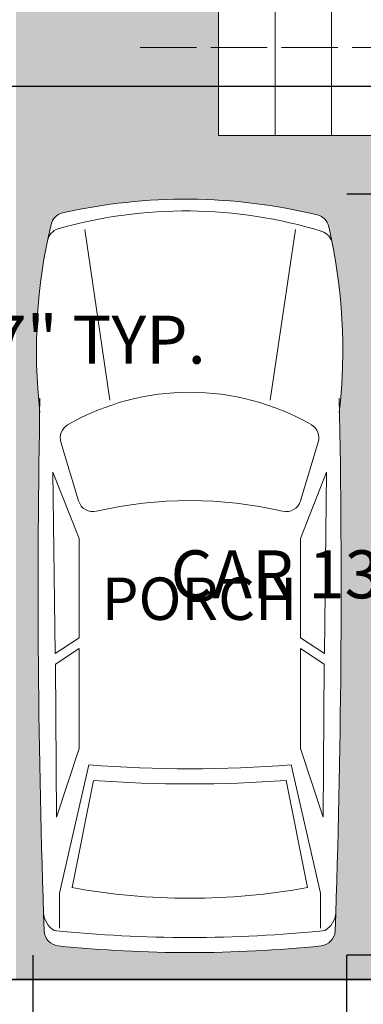
# Model space of a CAD drawing. Units: inches. Extents: x 1077 to 2505, y 1892 to 2728.
# Tile 22 of 26: x 2291 to 2364, y 2089 to 2298. Entities that reach past the tile are written whole.
import ezdxf

# ---------------------------------------------------------------- set-up
doc = ezdxf.new("R2010")
doc.units = ezdxf.units.IN
doc.linetypes.add('ACAD_ISO02W100', pattern=[15, 12, -3])
doc.layers.get('Defpoints').update_dxf_attribs({"color": 220, "linetype": 'ACAD_ISO02W100'})
for name, color, linetype, lineweight in [('A-ANNO-DIMS', 2, 'Continuous', 18), ('A-ANNO-STRS', 220, 'ACAD_ISO02W100', 13), ('A-AREA-IDEN', 7, 'Continuous', 18), ('A-FLOR-FIXT', 8, 'Continuous', 13), ('A-FLOR-STRS', 7, 'Continuous', 18), ('A-FURNITURE', 251, 'Continuous', 5), ('A-SITE-VEHI', 8, 'Continuous', 13), ('A_TEXT_SMALL', 18, 'Continuous', 13), ('WALL', 7, 'Continuous', 35)]:
    doc.layers.add(name, color=color, linetype=linetype, lineweight=lineweight)
doc.layers.add('A-FLOR-PATT', color=254, linetype='Continuous', lineweight=9, true_color=0xd7ebd2)
doc.styles.get("Standard").update_dxf_attribs({"font": 'arial.ttf'})
doc.dimstyles.get("Standard").update_dxf_attribs({"dimtxt": 10.18, "dimasz": 0.18, "dimexe": 0.18, "dimexo": 0.0625, "dimgap": 0.09, "dimtad": 0, "dimtih": 1, "dimtoh": 1, "dimdec": 0, "dimzin": 0, "dimdsep": 46, "dimlunit": 3, "dimtxsty": 'Standard', "dimcen": 0.09, "dimadec": 0, "dimazin": 0, "dimtfac": 1, "dimtdec": 0, "dimtofl": 0, "dimtmove": 0, "dimatfit": 3, "dimfxl": 1, "dimtolj": 1, "dimtzin": 0, "dimarcsym": 0})

# ---------------------------------------------------------------- blocks, each defined once
blk = doc.blocks.new('CAR')
at = {"layer": 'A-FURNITURE'}
for p, q in [((2677.91, 1665.57), (2683.24, 1629.33)), ((2722.63, 1665.57), (2717.3, 1629.33)), ((2672.85, 1620.44), (2676.61, 1608)), ((2727.48, 1620.44), (2723.73, 1608)), ((2671.15, 1614.07), (2676.73, 1600.01)), ((2671.63, 1575.61), (2671.15, 1614.07)), ((2729.25, 1614.07), (2723.67, 1600.01)), ((2728.77, 1575.61), (2729.25, 1614.07)), ((2676.73, 1600.01), (2676.73, 1578.97)), ((2723.67, 1600.01), (2723.67, 1578.97)), ((2676.73, 1578.97), (2671.63, 1575.61)), ((2723.67, 1578.97), (2728.77, 1575.61)), ((2676.73, 1576.71), (2671.66, 1573.38)), ((2676.73, 1576.71), (2676.73, 1555.46)), ((2723.67, 1576.71), (2723.67, 1555.46)), ((2723.67, 1576.71), (2728.74, 1573.38)), ((2671.9, 1540.91), (2671.66, 1573.38)), ((2728.49, 1540.91), (2728.74, 1573.38)), ((2676.73, 1555.46), (2671.9, 1540.91)), ((2723.67, 1555.46), (2728.49, 1540.91)), ((2678.77, 1552.01), (2672.52, 1524.85)), ((2721.71, 1552.02), (2727.96, 1524.85)), ((2675.22, 1526.01), (2679.74, 1548.74)), ((2725.17, 1526.01), (2720.66, 1548.74)), ((2672.52, 1524.85), (2672.52, 1517.39)), ((2727.96, 1524.85), (2727.96, 1517.39))]:
    blk.add_line(p, q, dxfattribs=at)
for centre, radius, start, end in [((2699.3, 1552.83), 119.14, 76.3976, 102.667), ((2674, 1665.84), 3.34, 104.3452, 166.6607), ((2699.3, 1570.19), 99.28, 73.0347, 105.8141), ((2726.43, 1665.41), 3.34, 13.1156, 74.5941), ((2783.1, 1639.97), 115.47, 166.6607, 186.5655), ((2617.23, 1639.97), 115.47, 353.4345, 13.1156), ((2673.27, 1662.52), 3.34, 107.8179, 168.3942), ((2727.17, 1661.99), 3.34, 11.3249, 70.8826), ((2700.17, 1579.09), 51.94, 60.0774, 119.9226), ((4741.11, 1589.62), 2073.11, 178.89024, 182.01225), ((659.22, 1589.62), 2073.11, 357.98775, 1.10976), ((2675.91, 1621.37), 3.2, 121.1455, 196.7984), ((2724.42, 1621.37), 3.2, 343.2016, 58.8545), ((2679.67, 1608.92), 3.2, 196.7984, 283.6631), ((2700.17, 1519.83), 88.22, 77.0683, 102.9317), ((2720.66, 1608.92), 3.2, 256.3369, 343.2016), ((2700.16, 1829.45), 278.26, 265.5919, 274.4407), ((2700.17, 1827.63), 279.65, 265.7971, 274.2029), ((2700.17, 1663.47), 139.72, 259.6897, 280.3103), ((2674.03, 1521.04), 4.9, 184.3987, 237.5288), ((2726.3, 1521.04), 4.9, 302.4712, 355.6013), ((2672.62, 1516.95), 3.34, 182.1119, 263.4899), ((2700.17, 1791.26), 275.86, 264.0142, 275.9858), ((2727.71, 1516.95), 3.34, 276.5101, 357.8881), ((2700.17, 1790.18), 277.96, 264.2342, 275.7658)]:
    blk.add_arc(centre, radius, start, end, dxfattribs=at)
blk = doc.blocks.new('reh-flat-2')
at = {"layer": 'A_TEXT_SMALL'}
for p, q in [((486053827.2, -394630231.2), (486054182.4, -394629799.8)), ((486054182.4, -394629799.8), (486054596.6, -394630140.9)), ((486053979.5, -394630126.3), (486054157.1, -394629910.6)), ((486054228.6, -394629903.6), (486054483.5, -394630113.5)), ((486054596.6, -394630140.9), (486054241.4, -394630572.3)), ((486054241.3, -394630407.7), (486053986.4, -394630197.8)), ((486054490.4, -394630185), (486054312.8, -394630400.7)), ((486054241.4, -394630572.3), (486053827.2, -394630231.2))]:
    blk.add_line(p, q, dxfattribs=at)
for centre, radius in [((486054234.9, -394630155.7), 38.1), ((486054004.1, -394630296.2), 20.1), ((486054072.7, -394630352.7), 20.1), ((486054141.4, -394630409.3), 20.1)]:
    blk.add_circle(centre, radius, dxfattribs=at)
for centre, start, end in [((486054196.3, -394629942.9), 50.5305, 140.5305), ((486054018.7, -394630158.5), 140.5305, 230.5305), ((486054451.2, -394630152.8), 320.5305, 50.5305), ((486054273.6, -394630368.4), 230.5305, 320.5305)]:
    blk.add_arc(centre, 50.8, start, end, dxfattribs=at)
blk = doc.blocks.new('STAIR-PLAN-RETURN')
for p, q in [((0, 163.08), (0, 127.08)), ((12, 163.08), (12, 127.08)), ((24, 163.08), (24, 127.08)), ((36, 163.08), (36, 0)), ((36, 163.08), (36, 127.08)), ((0, 127.08), (72, 127.08)), ((36, 115.08), (72, 115.08)), ((36, 103.08), (72, 103.08)), ((36, 91.08), (72, 91.08)), ((36, 79.08), (72, 79.08)), ((36, 67.08), (72, 67.08)), ((36, 55.08), (72, 55.08)), ((36, 43.08), (72, 43.08)), ((36, 31.08), (72, 31.08)), ((36, 19.08), (72, 19.08)), ((36, 7.08), (72, 7.08)), ((72, 0), (36, 0))]:
    blk.add_line(p, q)
blk = doc.blocks.new('STAIR-DIRECTION')
for p, q in [((0, 107.9), (70.51, 107.9)), ((70.51, 107.9), (70.51, 0)), ((70.51, 0), (75.75, 12.88)), ((75.75, 12.88), (70.51, 0.8)), ((70.51, 0.8), (65.28, 12.48)), ((65.28, 12.48), (70.51, 1.21))]:
    blk.add_line(p, q)
blk = doc.blocks.new('*D40')
at = {"layer": 'A-ANNO-DIMS', "color": 0, "lineweight": -2, "transparency": 16777216}
for p, q in [((2203.23, 2225.22), (2203.23, 2230.01)), ((2203.41, 2229.83), (2234.16, 2229.83)), ((2234.34, 2225.22), (2234.34, 2230.01)), ((2234.34, 2229.83), (2234.52, 2229.83))]:
    blk.add_line(p, q, dxfattribs=at)
at = {"layer": 'A-ANNO-DIMS', "color": 0, "transparency": 16777216}
for points in [[(2203.41, 2229.86), (2203.41, 2229.8), (2203.23, 2229.83)], [(2234.16, 2229.86), (2234.16, 2229.8), (2234.34, 2229.83)]]:
    blk.add_solid(points, dxfattribs=at)
at = {"layer": 'Defpoints', "color": 0, "transparency": 16777216}
for p in [(2234.34, 2229.83), (2203.23, 2225.16), (2234.34, 2225.16)]:
    blk.add_point(p, dxfattribs=at)
at = {"layer": 'A-ANNO-DIMS', "color": 0, "transparency": 16777216, "insert": (2282.74, 2229.83), "char_height": 10.18, "attachment_point": 5}
blk.add_mtext('\\A1;HOB 2\'-7" TYP.', dxfattribs=at)
blk = doc.blocks.new('*D46')
at = {"layer": 'A-ANNO-DIMS', "color": 0, "lineweight": -2, "transparency": 16777216}
for p, q in [((2289.89, 2308.17), (2289.89, 2302.65)), ((2325.89, 2308.17), (2325.89, 2302.65)), ((2289.89, 2302.83), (2289.71, 2302.83)), ((2325.71, 2302.83), (2290.07, 2302.83))]:
    blk.add_line(p, q, dxfattribs=at)
at = {"layer": 'A-ANNO-DIMS', "color": 0, "transparency": 16777216}
for points in [[(2290.07, 2302.86), (2290.07, 2302.8), (2289.89, 2302.83)], [(2325.71, 2302.86), (2325.71, 2302.8), (2325.89, 2302.83)]]:
    blk.add_solid(points, dxfattribs=at)
at = {"layer": 'Defpoints', "color": 0, "transparency": 16777216}
for p in [(2289.89, 2308.23), (2325.89, 2308.23), (2289.89, 2302.83)]:
    blk.add_point(p, dxfattribs=at)
at = {"layer": 'A-ANNO-DIMS', "color": 0, "transparency": 16777216, "insert": (2209.47, 2302.83), "char_height": 10.18, "attachment_point": 5}
blk.add_mtext('\\A1;DOOR SWING 3\'-0" TYP.', dxfattribs=at)
blk = doc.blocks.new('*D56')
at = {"layer": 'A-ANNO-DIMS', "color": 0, "lineweight": -2, "transparency": 16777216}
for p, q in [((2360.05, 2260.72), (2384.37, 2260.72)), ((2384.19, 2260.54), (2384.19, 2185.41)), ((2384.19, 2099.57), (2384.19, 2174.7)), ((2360.05, 2099.39), (2384.37, 2099.39))]:
    blk.add_line(p, q, dxfattribs=at)
at = {"layer": 'A-ANNO-DIMS', "color": 0, "transparency": 16777216}
for points in [[(2384.16, 2260.54), (2384.22, 2260.54), (2384.19, 2260.72)], [(2384.16, 2099.57), (2384.22, 2099.57), (2384.19, 2099.39)]]:
    blk.add_solid(points, dxfattribs=at)
at = {"layer": 'Defpoints', "color": 0, "transparency": 16777216}
for p in [(2359.99, 2260.72), (2384.19, 2260.72), (2359.99, 2099.39)]:
    blk.add_point(p, dxfattribs=at)
at = {"layer": 'A-ANNO-DIMS', "color": 0, "transparency": 16777216, "insert": (2384.19, 2180.06), "char_height": 10.18, "attachment_point": 5}
blk.add_mtext('\\A1;CAR 13\'-5 1/2" TYP.', dxfattribs=at)
blk = doc.blocks.new('*D57')
at = {"layer": 'A-ANNO-DIMS', "color": 0, "lineweight": -2, "transparency": 16777216}
for p, q in [((2293.39, 2099.33), (2293.39, 2075.01)), ((2359.99, 2099.33), (2359.99, 2075.01)), ((2293.57, 2075.19), (2359.81, 2075.19)), ((2359.99, 2075.19), (2360.17, 2075.19))]:
    blk.add_line(p, q, dxfattribs=at)
at = {"layer": 'A-ANNO-DIMS', "color": 0, "transparency": 16777216}
for points in [[(2293.57, 2075.22), (2293.57, 2075.16), (2293.39, 2075.19)], [(2359.81, 2075.22), (2359.81, 2075.16), (2359.99, 2075.19)]]:
    blk.add_solid(points, dxfattribs=at)
at = {"layer": 'Defpoints', "color": 0, "transparency": 16777216}
for p in [(2293.39, 2099.39), (2359.99, 2099.39), (2359.99, 2075.19)]:
    blk.add_point(p, dxfattribs=at)
at = {"layer": 'A-ANNO-DIMS', "color": 0, "transparency": 16777216, "insert": (2403.15, 2075.19), "char_height": 10.18, "attachment_point": 5}
blk.add_mtext('\\A1;5\'-6 1/2" TYP.', dxfattribs=at)
blk = doc.blocks.new('*D63')
at = {"layer": 'A-ANNO-DIMS', "color": 0, "lineweight": -2, "transparency": 16777216}
for p, q in [((2035.85, 2094.07), (2035.85, 2065.11)), ((2413.85, 2094.07), (2413.85, 2065.11)), ((2036.03, 2065.29), (2207.27, 2065.29)), ((2413.67, 2065.29), (2242.42, 2065.29))]:
    blk.add_line(p, q, dxfattribs=at)
at = {"layer": 'A-ANNO-DIMS', "color": 0, "transparency": 16777216}
for points in [[(2036.03, 2065.32), (2036.03, 2065.26), (2035.85, 2065.29)], [(2413.67, 2065.32), (2413.67, 2065.26), (2413.85, 2065.29)]]:
    blk.add_solid(points, dxfattribs=at)
at = {"layer": 'Defpoints', "color": 0, "transparency": 16777216}
for p in [(2035.85, 2094.14), (2413.85, 2094.14), (2413.85, 2065.29)]:
    blk.add_point(p, dxfattribs=at)
at = {"layer": 'A-ANNO-DIMS', "color": 0, "transparency": 16777216, "insert": (2224.85, 2065.29), "char_height": 10.18, "attachment_point": 5}
blk.add_mtext('\\A1;31\'-6"', dxfattribs=at)
blk = doc.blocks.new('*D69')
at = {"layer": 'A-ANNO-DIMS', "color": 0, "lineweight": -2, "transparency": 16777216}
for p, q in [((2263.27, 2262.49), (2263.27, 2065.11)), ((2285.18, 2262.49), (2285.18, 2065.11)), ((2263.45, 2065.29), (2285, 2065.29)), ((2285.18, 2065.29), (2285.36, 2065.29))]:
    blk.add_line(p, q, dxfattribs=at)
at = {"layer": 'A-ANNO-DIMS', "color": 0, "transparency": 16777216}
for points in [[(2263.45, 2065.32), (2263.45, 2065.26), (2263.27, 2065.29)], [(2285, 2065.32), (2285, 2065.26), (2285.18, 2065.29)]]:
    blk.add_solid(points, dxfattribs=at)
at = {"layer": 'Defpoints', "color": 0, "transparency": 16777216}
for p in [(2263.27, 2262.55), (2285.18, 2262.55), (2285.18, 2065.29)]:
    blk.add_point(p, dxfattribs=at)
at = {"layer": 'A-ANNO-DIMS', "color": 0, "transparency": 16777216, "insert": (2302.45, 2065.29), "char_height": 10.18, "attachment_point": 5}
blk.add_mtext('\\A1;1\'-10"', dxfattribs=at)
blk = doc.blocks.new('*D72')
at = {"layer": 'A-ANNO-DIMS', "color": 0, "lineweight": -2, "transparency": 16777216}
for p, q in [((2280.86, 2313.12), (2442.88, 2313.12)), ((2442.7, 2312.94), (2442.7, 2303.7)), ((2442.7, 2283.76), (2442.7, 2292.99)), ((2285.24, 2283.58), (2442.88, 2283.58))]:
    blk.add_line(p, q, dxfattribs=at)
at = {"layer": 'A-ANNO-DIMS', "color": 0, "transparency": 16777216}
for points in [[(2442.67, 2312.94), (2442.73, 2312.94), (2442.7, 2313.12)], [(2442.67, 2283.76), (2442.73, 2283.76), (2442.7, 2283.58)]]:
    blk.add_solid(points, dxfattribs=at)
at = {"layer": 'Defpoints', "color": 0, "transparency": 16777216}
for p in [(2280.8, 2313.12), (2285.18, 2283.58), (2442.7, 2283.58)]:
    blk.add_point(p, dxfattribs=at)
at = {"layer": 'A-ANNO-DIMS', "color": 0, "transparency": 16777216, "insert": (2442.7, 2298.35), "char_height": 10.18, "attachment_point": 5}
blk.add_mtext('\\A1;2\'-5 1/2"', dxfattribs=at)

msp = doc.modelspace()

# ---------------------------------------------------------------- hatches: boundary and pattern name
at = {"layer": 'A-FLOR-PATT', "transparency": 33554559}
h = msp.add_hatch(color=256, dxfattribs=at)
h.dxf.hatch_style = 1
h.paths.add_polyline_path([(2252.85, 2583.14), (2232.15, 2583.14), (2208.15, 2583.17), (2208.15, 2583.14), (2186.85, 2583.14), (2186.85, 2486.14), (2186.85, 2475.14), (2182.85, 2475.14), (2182.85, 2521.11), (2164.84, 2521.11), (2164.84, 2583.14), (2126.63, 2583.14), (2078.63, 2583.13), (2078.63, 2583.14), (2044.85, 2583.14), (2044.85, 2439.14), (2146.85, 2439.14), (2146.85, 2435.14), (2120.85, 2435.14), (2044.85, 2435.14), (2044.85, 2401), (2044.85, 2401), (2044.85, 2377), (2044.85, 2377), (2044.85, 2313.14), (2116.85, 2313.14), (2116.85, 2405.14), (2120.85, 2405.14), (2120.85, 2313.14), (2146.85, 2313.14), (2146.85, 2312.21), (2182.85, 2312.21), (2182.85, 2313.14), (2186.85, 2313.14), (2186.85, 2312.21), (2222.85, 2312.21), (2222.85, 2313.14), (2289.85, 2313.14), (2289.85, 2094.14), (2404.85, 2094.14), (2404.85, 2146.06), (2368.85, 2146.06), (2368.85, 2273.14), (2332.85, 2273.14), (2332.85, 2309.14), (2325.85, 2309.14), (2325.85, 2313.14), (2404.85, 2313.14), (2404.85, 2354.2), (2404.85, 2402.2), (2404.85, 2435.14), (2292.85, 2435.14), (2292.85, 2439.14), (2333.66, 2439.14), (2333.66, 2457.16), (2404.85, 2457.16), (2404.85, 2583.14), (2356.85, 2583.14), (2356.85, 2592.14), (2404.85, 2592.14), (2404.85, 2648.14), (2375.5, 2648.14), (2375.5, 2648.03), (2351.47, 2648.03), (2351.47, 2648.14), (2326.85, 2648.14), (2326.85, 2583.14), (2256.85, 2583.14), (2256.85, 2435.14), (2182.85, 2435.14), (2182.85, 2439.14), (2186.85, 2439.14), (2252.85, 2439.14), (2252.85, 2486.14), (2216.85, 2486.14), (2216.85, 2490.14), (2252.85, 2490.14)])
h.paths.add_polyline_path([(2214.97, 2488.05), (2212.97, 2488.05), (2212.97, 2487.05, 0.414214), (2213.97, 2486.05), (2201.97, 2486.05), (2201.97, 2483.04), (2200.58, 2483.04), (2200.58, 2486.05), (2187.97, 2486.05, -0.414214), (2186.97, 2487.05), (2186.97, 2490.05), (2188.97, 2490.05), (2188.97, 2516.05, -0.446908)], flags=16)
h.paths.add_polyline_path([(2162.4, 2565.16), (2146.2, 2565.16), (2146.2, 2581.36), (2162.4, 2581.36)], flags=16)
h.paths.add_polyline_path([(2161.5, 2566.06), (2147.1, 2566.06), (2147.1, 2580.46), (2161.5, 2580.46)], flags=0)
h.paths.add_polyline_path([(2145.3, 2506.66, -0.414214), (2144.4, 2505.76), (2122.45, 2505.76), (2081.4, 2505.76, -0.414214), (2080.5, 2506.66), (2080.5, 2563.14), (2080.5, 2577.72), (2080.5, 2581.36), (2145.3, 2581.36), (2145.3, 2577.72), (2144.4, 2577.72, -0.414214), (2145.3, 2576.82)], flags=16)
h.paths.add_polyline_path([(2150.3, 2575.03, -1), (2158.24, 2575.03, -1)], flags=0)
h.paths.add_polyline_path([(2150.64, 2575.03, -1), (2157.89, 2575.03, -1)], flags=0)
h.paths.add_polyline_path([(2180.11, 2468.19), (2180.11, 2437.69), (2180.36, 2436.69), (2180.36, 2437.69), (2179.11, 2437.69), (2179.11, 2468.17, 0.404641), (2149.61, 2437.69), (2149.36, 2436.69, -0.414214), (2148.86, 2436.19), (2148.36, 2436.19), (2148.36, 2435.69, -0.414214), (2147.86, 2435.19), (2146.86, 2435.19), (2146.86, 2440.19), (2147.86, 2440.19, -0.414214), (2148.36, 2439.69), (2148.36, 2439.19), (2148.86, 2439.19, -0.414214), (2149.36, 2438.69), (2149.61, 2437.69, -0.414214)], flags=16)
h.paths.add_polyline_path([(2145.14, 2554.26, 0.292232), (2136.49, 2542.78, 0.052719), (2081.25, 2554.26), (2080.6, 2554.26), (2080.6, 2563.14), (2081.25, 2563.14), (2102.73, 2563.14, -0.117785), (2103.09, 2563.91, -0.059418), (2112.19, 2573, -0.379859), (2114.6, 2572.86, -0.02509), (2118.73, 2569.3, -0.025935), (2122.97, 2573, -0.379859), (2125.38, 2572.86, -0.061767), (2134.84, 2563.41, -0.069393), (2135.14, 2563.14), (2145.14, 2563.14)], flags=0)
h.paths.add_polyline_path([(2120.79, 2554.26), (2117.88, 2554.26, -0.015371), (2115.33, 2552.11, -0.429576), (2112.69, 2552.04, -0.016036), (2110.01, 2554.26), (2080.6, 2554.26), (2080.6, 2560.4), (2104.1, 2560.4, 0.055344), (2112.69, 2552.04, 0.331768), (2114.84, 2551.72, 0.027343), (2119.32, 2555.62, 0.00919)], flags=0)
h.paths.add_polyline_path([(2152.88, 2574.32), (2154.19, 2575.07), (2154.19, 2576.58, 0.399698), (2152.71, 2575.03, 0.119004)], flags=0)
h.paths.add_polyline_path([(2152.53, 2575.03, -1), (2156, 2575.03, -1)], flags=0)
h.paths.add_polyline_path([(2154.27, 2574.94), (2154.34, 2574.98), (2154.34, 2575.07), (2154.3, 2575.09), (2154.23, 2574.96)], flags=0)
h.paths.add_polyline_path([(2259.6, 2468.17, -0.414214), (2290.1, 2437.67), (2290.35, 2438.67), (2290.1, 2437.67, 0.404641), (2260.6, 2468.15), (2260.6, 2437.67), (2259.35, 2437.67), (2259.35, 2436.67, -0.414214), (2258.85, 2436.17), (2258.35, 2436.17), (2258.35, 2435.67, -0.414214), (2257.85, 2435.17), (2256.85, 2435.17), (2256.85, 2440.17), (2257.85, 2440.17, -0.414214), (2258.35, 2439.67), (2258.35, 2439.17), (2258.85, 2439.17, -0.414214), (2259.35, 2438.67)], flags=16)
h.paths.add_polyline_path([(2327.48, 2541.19, -0.414214), (2328.38, 2542.09), (2384.85, 2542.09), (2399.43, 2542.09), (2403.08, 2542.09), (2403.08, 2477.29), (2399.43, 2477.29), (2399.43, 2478.19, -0.414214), (2398.53, 2477.29), (2328.38, 2477.29, -0.414214), (2327.48, 2478.19), (2327.48, 2500.14)], flags=16)
h.paths.add_polyline_path([(2340.38, 2542.09, 0.253465), (2337.43, 2532.13, 0.2538), (2327.47, 2529.17)], flags=16)
h.paths.add_polyline_path([(2080.5, 2518.67, 0.253465), (2090.46, 2515.72, 0.2538), (2093.42, 2505.75)], flags=16)
h.paths.add_polyline_path([(2327.09, 2584.7), (2327.09, 2587.7), (2329.09, 2587.7), (2329.09, 2613.7, -0.01951), (2331.09, 2613.66), (2331.09, 2585.7), (2331.09, 2584.7, -0.414214), (2330.09, 2583.7), (2328.09, 2583.7, -0.414214)], flags=16)
h.paths.add_polyline_path([(2239.78, 2404.11), (2252.36, 2404.11), (2252.36, 2405.72), (2239.78, 2405.72)], flags=16)
h.paths.add_polyline_path([(2237.26, 2403.16), (2237.26, 2395.8), (2237.82, 2395.8), (2237.82, 2402.03, -0.41429), (2238.38, 2402.59), (2253.79, 2402.59, -0.414213), (2254.35, 2402.03), (2254.35, 2395.8), (2254.91, 2395.8), (2254.91, 2403.16)], flags=16)
h.paths.add_polyline_path([(2120.69, 2434.12), (2120.69, 2432.12, -0.414214), (2119.69, 2431.12), (2118.69, 2431.12), (2090.73, 2431.12, 0.400854), (2116.69, 2407.02), (2116.69, 2407.12), (2118.69, 2407.12, -0.446908), (2090.69, 2433.12), (2116.69, 2433.12), (2116.69, 2435.12), (2119.69, 2435.12, -0.414214)], flags=16)
h.paths.add_polyline_path([(2262.11, 2404.11), (2274.69, 2404.11), (2274.69, 2405.72), (2262.11, 2405.72)], flags=16)
h.paths.add_polyline_path([(2259.59, 2403.16), (2262.11, 2404.11), (2274.69, 2404.11), (2277.24, 2403.16)], flags=16)
h.paths.add_polyline_path([(2289.58, 2389.14), (2289.58, 2376.57), (2291.19, 2376.57), (2291.19, 2389.14)], flags=16)
h.paths.add_polyline_path([(2288.62, 2391.67), (2281.15, 2391.67), (2281.15, 2391.11), (2287.5, 2391.11, -0.41429), (2288.06, 2390.54), (2288.06, 2375.14, -0.414237), (2287.5, 2374.58), (2281.15, 2374.58), (2281.15, 2374.01), (2288.62, 2374.01)], flags=16)
h.paths.add_polyline_path([(2274.69, 2357.14), (2274.69, 2355.52), (2276.22, 2355.52, 0.414236), (2277.24, 2356.54), (2277.24, 2358.09)], flags=16)
h.paths.add_polyline_path([(2252.36, 2357.14), (2252.36, 2355.52), (2253.89, 2355.52, 0.414235), (2254.91, 2356.54), (2254.91, 2358.09)], flags=16)
h.paths.add_polyline_path([(2224.02, 2376.03), (2222.41, 2376.03), (2222.41, 2374.5, 0.414235), (2223.43, 2373.48), (2224.98, 2373.48)], flags=16)
h.paths.add_polyline_path([(2276.68, 2365.45), (2276.68, 2359.22, -0.41419), (2276.12, 2358.66), (2260.71, 2358.66, -0.414137), (2260.15, 2359.22), (2260.15, 2365.45), (2254.35, 2365.45), (2254.35, 2359.22, -0.414189), (2253.79, 2358.66), (2238.38, 2358.66, -0.414137), (2237.82, 2359.22), (2237.82, 2365.45)], flags=16)
h.paths.add_polyline_path([(2079.6, 2565.16), (2063.4, 2565.16), (2063.4, 2581.36), (2079.6, 2581.36)], flags=16)
h.paths.add_polyline_path([(2078.7, 2566.06), (2064.3, 2566.06), (2064.3, 2580.46), (2078.7, 2580.46)], flags=0)
h.paths.add_polyline_path([(2339.31, 2583.7), (2339.31, 2586.71), (2340.7, 2586.71), (2340.7, 2583.7), (2342.09, 2583.7), (2342.09, 2580.7), (2340.7, 2580.7), (2340.7, 2583.7)], flags=16)
h.paths.add_polyline_path([(2123.69, 2421.51), (2123.69, 2420.12), (2120.69, 2420.12), (2120.69, 2421.51), (2117.68, 2421.51), (2117.68, 2422.89), (2120.69, 2422.89), (2120.69, 2421.51)], flags=16)
h.paths.add_polyline_path([(2067.57, 2575.03, -1), (2075.51, 2575.03, -1)], flags=0)
h.paths.add_polyline_path([(2067.92, 2575.03, -1), (2075.17, 2575.03, -1)], flags=0)
h.paths.add_polyline_path([(2070.16, 2574.32), (2071.47, 2575.07), (2071.47, 2576.58, 0.399698), (2069.99, 2575.03, 0.119004)], flags=0)
h.paths.add_polyline_path([(2069.81, 2575.03, -1), (2073.28, 2575.03, -1)], flags=0)
h.paths.add_polyline_path([(2071.54, 2574.94), (2071.62, 2574.89), (2071.62, 2574.98)], flags=0)
h.paths.add_polyline_path([(2364.5, 2486.1, 0.052719), (2375.98, 2541.34), (2375.98, 2541.99), (2384.85, 2541.99), (2384.85, 2541.34), (2384.85, 2519.86, -0.117785), (2385.62, 2519.51, -0.059418), (2394.72, 2510.41, -0.379859), (2394.58, 2507.99, -0.02509), (2391.01, 2503.87, -0.025935), (2394.72, 2499.62, -0.379859), (2394.58, 2497.21, -0.061767), (2385.12, 2487.75, -0.069393), (2384.85, 2487.45), (2384.85, 2477.45), (2375.98, 2477.45, 0.292232)], flags=0)
h.paths.add_polyline_path([(2373.75, 2509.9, -0.016036), (2375.98, 2512.58), (2375.98, 2541.99), (2382.12, 2541.99), (2382.12, 2518.49, 0.055344), (2373.75, 2509.9, 0.331768), (2373.44, 2507.75, 0.027343), (2377.33, 2503.27, 0.00919), (2375.98, 2501.8), (2375.98, 2504.71, -0.015371), (2373.82, 2507.26, -0.429576)], flags=0)
h.paths.add_polyline_path([(2356.95, 2631.48, -0.171636), (2360.13, 2636.99), (2360.13, 2639.35), (2356, 2639.35, -0.414214), (2355.01, 2640.34), (2355.01, 2646.64, -0.414214), (2356, 2647.62), (2372.14, 2647.62, -0.414214), (2373.13, 2646.64), (2373.13, 2640.34, -0.414214), (2372.14, 2639.35), (2368.01, 2639.35), (2368.01, 2636.99, -0.171636), (2371.2, 2631.48, -0.258205), (2366.63, 2620.45), (2361.51, 2620.45, -0.258205)], flags=16)
h.paths.add_polyline_path([(2358.52, 2631.48, -0.171636), (2361.71, 2636.99), (2366.43, 2636.99, -0.171636), (2369.62, 2631.48, -0.210384), (2366.67, 2622), (2361.47, 2622, -0.210384)], flags=0)
h.paths.add_polyline_path([(2386.88, 2542.99), (2386.88, 2559.19), (2403.08, 2559.19), (2403.08, 2542.99)], flags=16)
h.paths.add_polyline_path([(2387.78, 2543.89), (2387.78, 2558.29), (2402.18, 2558.29), (2402.18, 2543.89)], flags=0)
h.paths.add_polyline_path([(2392.77, 2551.05, -1), (2400.71, 2551.05, -1)], flags=0)
h.paths.add_polyline_path([(2393.11, 2551.05, -1), (2400.37, 2551.05, -1)], flags=0)
h.paths.add_polyline_path([(2386.88, 2476.39), (2403.08, 2476.39), (2403.08, 2460.19), (2386.88, 2460.19)], flags=16)
h.paths.add_polyline_path([(2398.48, 2550.97), (2398.3, 2550.97, -0.544606), (2396.03, 2549.66), (2395.94, 2549.51, 0.547962)], flags=0)
h.paths.add_polyline_path([(2387.78, 2475.49), (2402.18, 2475.49), (2402.18, 2461.09), (2387.78, 2461.09)], flags=0)
h.paths.add_polyline_path([(2396.79, 2551.12), (2396.74, 2551.2), (2396.7, 2551.12)], flags=0)
h.paths.add_polyline_path([(2400.71, 2468.32, -1), (2392.77, 2468.32, -1)], flags=0)
h.paths.add_polyline_path([(2400.37, 2468.32, -1), (2393.11, 2468.32, -1)], flags=0)
h.paths.add_polyline_path([(2398.48, 2468.25), (2398.3, 2468.25, -0.544606), (2396.03, 2466.94), (2395.94, 2466.78, 0.547962)], flags=0)
h.paths.add_polyline_path([(2396.79, 2468.4), (2396.74, 2468.48), (2396.7, 2468.4)], flags=0)
h.paths.add_polyline_path([(2292.64, 2341.23, -0.414214), (2323.14, 2310.73), (2323.39, 2311.73), (2323.14, 2310.73, 0.404641), (2293.64, 2341.21), (2293.64, 2310.73), (2292.39, 2310.73), (2292.39, 2309.73, -0.414214), (2291.89, 2309.23), (2291.39, 2309.23), (2291.39, 2308.73, -0.414214), (2290.89, 2308.23), (2289.89, 2308.23), (2289.89, 2313.23), (2290.89, 2313.23, -0.414214), (2291.39, 2312.73), (2291.39, 2312.23), (2291.89, 2312.23, -0.414214), (2292.39, 2311.73)], flags=16)
h.paths.add_polyline_path([(2389.45, 2641.69), (2392.75, 2641.69), (2392.75, 2641.87), (2389.45, 2641.87)], flags=16)
edge = h.paths.add_edge_path(flags=16)
edge.add_arc((2393.3, 2638.65), 0.183, 270, 360)
edge.add_line((2393.49, 2638.65), (2393.49, 2645.8))
edge.add_line((2393.49, 2645.8), (2395.61, 2645.8))
edge.add_line((2395.61, 2645.8), (2395.61, 2647.8))
edge.add_line((2395.61, 2647.8), (2390.57, 2647.8))
edge.add_line((2390.57, 2647.8), (2390.57, 2645.8))
edge.add_line((2390.57, 2645.8), (2392.19, 2645.8))
edge.add_line((2392.19, 2645.8), (2392.19, 2644.98))
edge.add_line((2392.19, 2644.98), (2391.02, 2644.98))
edge.add_line((2391.02, 2644.98), (2391.02, 2645.8))
edge.add_line((2391.02, 2645.8), (2390.57, 2645.8))
edge.add_line((2390.57, 2645.8), (2390.57, 2647.8))
edge.add_line((2390.57, 2647.8), (2395.61, 2647.8))
edge.add_line((2395.61, 2647.8), (2395.61, 2647.32))
edge.add_line((2395.61, 2647.32), (2397.95, 2647.56))
edge.add_line((2397.95, 2647.56), (2397.95, 2647.8))
edge.add_line((2397.95, 2647.8), (2398.81, 2647.8))
edge.add_line((2398.81, 2647.8), (2398.81, 2647.23))
edge.add_line((2398.81, 2647.23), (2398.63, 2645.77))
edge.add_ellipse((2398.41, 2644.93), major_axis=(-1.08, 0), ratio=0.790849, start_angle=180, end_angle=255.2976, ccw=False)
edge.add_line((2399.49, 2644.93), (2399.49, 2644.36))
edge.add_ellipse((2398.41, 2644.36), major_axis=(-1.08, 0), ratio=0.790849, start_angle=0, end_angle=180, ccw=False)
edge.add_line((2397.32, 2644.36), (2397.33, 2644.85))
edge.add_ellipse((2398.41, 2644.93), major_axis=(-1.08, 0), ratio=0.790849, start_angle=284.7024, end_angle=364.0401, ccw=False)
edge.add_line((2398.1, 2645.73), (2398.1, 2647.23))
edge.add_line((2398.1, 2647.23), (2397.95, 2647.23))
edge.add_line((2397.95, 2647.23), (2395.61, 2646.99))
edge.add_line((2395.61, 2646.99), (2395.61, 2645.8))
edge.add_line((2395.61, 2645.8), (2393.49, 2645.8))
edge.add_line((2393.49, 2645.8), (2393.49, 2638.46))
edge.add_line((2393.49, 2638.46), (2393.3, 2638.46))
h.paths.add_polyline_path([(2353.64, 2256.32, -0.292371), (2356.22, 2253.81, -0.085148), (2358.52, 2214.83, -0.01331), (2357.59, 2104.48, -0.379287), (2354.54, 2101.26, -0.0502), (2298.86, 2101.26, -0.379287), (2295.81, 2104.48, -0.01331), (2294.88, 2214.83, -0.086132), (2297.28, 2254.24, -0.295116), (2299.9, 2256.76, -0.114238)], flags=16)
h.paths.add_polyline_path([(2352.48, 2211.82, -0.355389), (2354.02, 2208.08), (2350.26, 2195.63, -0.398275), (2346.44, 2193.45, 0.113332), (2306.96, 2193.45, -0.398275), (2303.14, 2195.63), (2299.38, 2208.08, -0.355394), (2300.92, 2211.82, -0.265725)], flags=0)
h.paths.add_polyline_path([(2297.68, 2201.7), (2303.26, 2187.65), (2303.26, 2166.61), (2298.16, 2163.24)], flags=0)
h.paths.add_polyline_path([(2355.78, 2201.7), (2355.31, 2163.24), (2350.2, 2166.61), (2350.2, 2187.65)], flags=0)
h.paths.add_polyline_path([(2303.26, 2164.35), (2303.26, 2143.1), (2298.44, 2128.54), (2298.19, 2161.01)], flags=0)
h.paths.add_polyline_path([(2350.2, 2164.35), (2355.28, 2161.01), (2355.03, 2128.54), (2350.2, 2143.1)], flags=0)
h.paths.add_polyline_path([(2347.2, 2136.38), (2351.71, 2113.65, -0.090102), (2301.76, 2113.63), (2306.27, 2136.37, 0.036636)], flags=0)
h.paths.add_polyline_path([(2304.86, 2165.32), (2354.76, 2165.32), (2354.76, 2183.87), (2304.86, 2183.87)], flags=8)
h.paths.add_polyline_path([(2053.76, 2360.82), (2103.97, 2360.82), (2103.97, 2394.41), (2053.76, 2394.41)], flags=24)
h.paths.add_polyline_path([(2153.41, 2366.23), (2211.12, 2366.23), (2211.12, 2399.82), (2153.41, 2399.82)], flags=24)
h.paths.add_polyline_path([(2258.04, 2477.83), (2327.95, 2477.83), (2327.95, 2511.42), (2258.04, 2511.42)], flags=24)
h.paths.add_polyline_path([(2182.1, 2454.46), (2252.27, 2454.46), (2252.27, 2473), (2182.1, 2473)], flags=24)
h.paths.add_polyline_path([(2192.4, 2537.41), (2246.99, 2537.41), (2246.99, 2571), (2192.4, 2571)], flags=24)
h.paths.add_polyline_path([(2083.07, 2465.98), (2152.99, 2465.98), (2152.99, 2499.56), (2083.07, 2499.56)], flags=24)

# ---------------------------------------------------------------- linework, layer by layer
at = {"layer": 'WALL'}
msp.add_line((2413.85, 2094.14), (2035.85, 2094.14), dxfattribs=at)

# ---------------------------------------------------------------- block references
at = {"layer": 'A-ANNO-STRS'}
msp.add_blockref('STAIR-DIRECTION', (2316.18, 2183.85), dxfattribs=at)
at = {"layer": 'A-FLOR-FIXT', "xscale": 0.0391972730482577, "yscale": 0.0391972730482577, "zscale": 0.0391972730482577, "rotation": 309.4694759622496}
msp.add_blockref('reh-flat-2', (-167395.5, 24542487.85), dxfattribs=at)
at = {"layer": 'A-FLOR-STRS'}
msp.add_blockref('STAIR-PLAN-RETURN', (2332.85, 2146.06), dxfattribs=at)
at = {"layer": 'A-SITE-VEHI'}
msp.add_blockref('CAR', (-373.47, 587.64), dxfattribs=at)

# ---------------------------------------------------------------- texts
at = {"layer": 'A-AREA-IDEN', "insert": (2308.08, 2179.39), "char_height": 9, "attachment_point": 1}
msp.add_mtext_dynamic_manual_height_columns('PORCH', width=128.1076, gutter_width=12.5, heights=[0], dxfattribs=at)

# ---------------------------------------------------------------- dimensions: what is measured, and where the dimension line sits
at = {"layer": 'A-ANNO-DIMS'}
for base, p1, p2, angle, text, picture, middle in [((2289.89, 2302.83), (2325.89, 2308.23), (2289.89, 2308.23), 180, 'DOOR SWING <> TYP.', '*D46', (2209.47, 2302.83)), ((2384.19, 2260.72), (2359.99, 2099.39), (2359.99, 2260.72), 90, 'CAR <> TYP.', '*D56', (2384.19, 2180.06))]:
    dim = msp.add_linear_dim(base=base, p1=p1, p2=p2, angle=angle, text=text, dimstyle='Standard', override={"dimdec": 1, "dimlfac": 1, "dimrnd": 0, "dimzin": 1, "dimdsep": 46, "dimlunit": 4, "dimfrac": 2}, dxfattribs=at)
    dim.commit()
    dim.dimension.update_dxf_attribs({"geometry": picture, "text_midpoint": middle})
dim = msp.add_linear_dim(base=(2442.7, 2283.58), p1=(2280.8, 2313.12), p2=(2285.18, 2283.58), angle=90, dimstyle='Standard', override={"dimdec": 1, "dimlfac": 1, "dimrnd": 0, "dimzin": 1, "dimdsep": 46, "dimlunit": 4, "dimfrac": 2}, dxfattribs=at)
dim.commit()
dim.dimension.update_dxf_attribs({"geometry": '*D72', "text_midpoint": (2442.7, 2298.35)})
for base, p1, p2, picture, middle in [((2285.18, 2065.29), (2263.27, 2262.55), (2285.18, 2262.55), '*D69', (2302.45, 2065.29)), ((2413.85, 2065.29), (2035.85, 2094.14), (2413.85, 2094.14), '*D63', (2224.85, 2065.29))]:
    dim = msp.add_linear_dim(base=base, p1=p1, p2=p2, dimstyle='Standard', override={"dimdec": 1, "dimlfac": 1, "dimrnd": 0, "dimzin": 1, "dimdsep": 46, "dimlunit": 4, "dimfrac": 2}, dxfattribs=at)
    dim.commit()
    dim.dimension.update_dxf_attribs({"geometry": picture, "text_midpoint": middle})
for base, p1, p2, text, picture, middle in [((2234.34, 2229.83), (2203.23, 2225.16), (2234.34, 2225.16), 'HOB <> TYP.', '*D40', (2282.74, 2229.83)), ((2359.99, 2075.19), (2293.39, 2099.39), (2359.99, 2099.39), '<> TYP.', '*D57', (2403.15, 2075.19))]:
    dim = msp.add_linear_dim(base=base, p1=p1, p2=p2, text=text, dimstyle='Standard', override={"dimdec": 1, "dimlfac": 1, "dimrnd": 0, "dimzin": 1, "dimdsep": 46, "dimlunit": 4, "dimfrac": 2}, dxfattribs=at)
    dim.commit()
    dim.dimension.update_dxf_attribs({"geometry": picture, "text_midpoint": middle})

doc.saveas('drawing.dxf')
